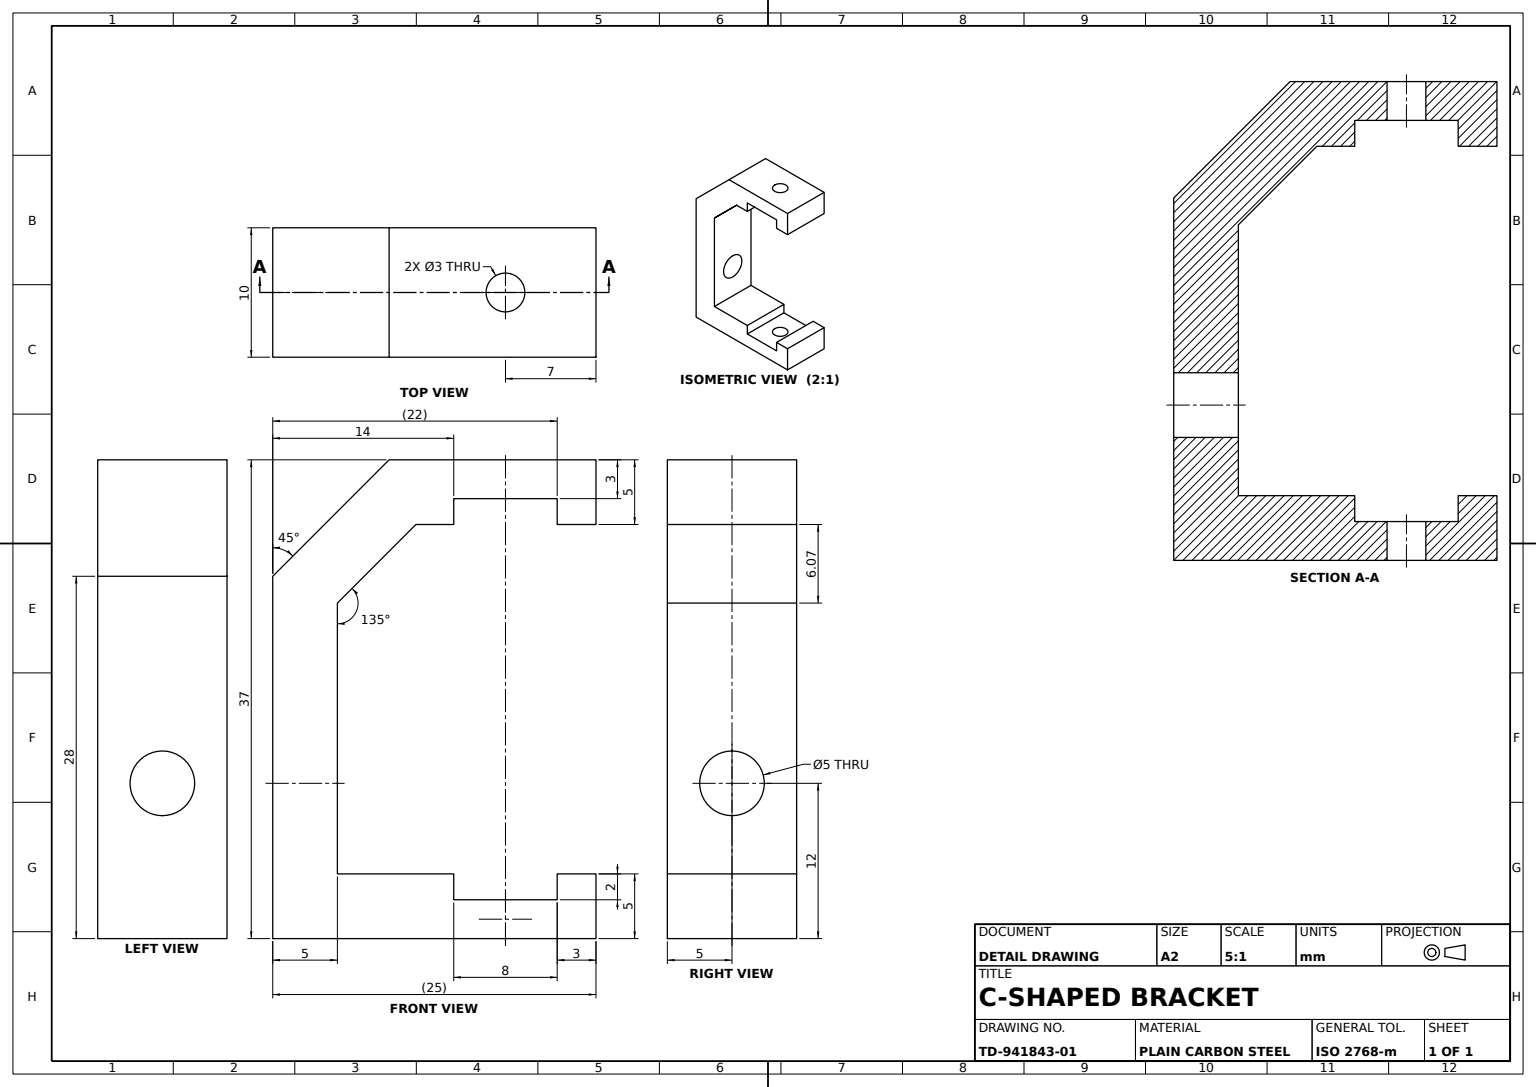
SolidWorks part; units mm, degrees
material "Plain Carbon Steel"
ref_plane "Front Plane" through (0, 0, 0) normal (0, 0, 1) x (1, 0, 0)
ref_plane "Top Plane" through (0, 0, 0) normal (0, 1, 0) x (1, 0, 0)
ref_plane "Right Plane" through (0, 0, 0) normal (1, 0, 0) x (0, 0, -1)
sketch "C Profile Sketch" plane through (0, 0, 0) normal (0, 0, 1) x (1, 0, 0)
  line L0 (0, 0) -> (0, 28)
  line L1 (0, 28) -> (9, 37)
  line L2 (9, 37) -> (25, 37)
  line L3 (25, 37) -> (25, 32)
  line L4 (25, 32) -> (22, 32)
  line L5 (22, 32) -> (22, 34)
  line L6 (22, 34) -> (14, 34)
  line L7 (14, 34) -> (14, 32)
  line L8 (14, 32) -> (11.0711, 32)
  line L9 (11.0711, 32) -> (5, 25.9289)
  line L10 (5, 25.9289) -> (5, 5)
  line L11 (5, 5) -> (14, 5)
  line L12 (14, 5) -> (14, 3)
  line L13 (14, 3) -> (22, 3)
  line L14 (22, 3) -> (22, 5)
  line L15 (22, 5) -> (25, 5)
  line L16 (25, 5) -> (25, 0)
  line L17 (25, 0) -> (0, 0)
  dimension "D1" = 28
  dimension "D2" = 45
  dimension "D3" = 5
  dimension "D4" = 2
  dimension "D5" = 5
  dimension "D6" = 8
  dimension "D7" = 3
  dimension "D8" = 5
  dimension "D9" = 37
  dimension "D10" = 3
  dimension "D11" = 8
  dimension "D12" = 5
  dimension "D13" = 5
  dimension "D14" = 2
  dimension "D15" = 25
  dimension "D16" = 25
  dimension "D17" = 5
extrude "C Bracket Body" add sketch "C Profile Sketch" along normal mid plane 10
sketch "Flange Hole Sketch" plane through (0, 34, 0) normal (0, -1, 0) x (1, 0, 0)
  line L0 (22, 5) -> (22, -5) construction
  line L5 (14, -5) -> (22, -5) construction
  line L6 (0, -5) -> (25, -5) construction
  line L8 (25, 5) -> (25, -5) construction
  circle A0 centre (18, 0) radius 1.5
  dimension "D1" = 3
  dimension "D2" = 5
  dimension "D3" = 7
  dimension "D4" = 4
  dimension "D5" = 5
extrude "Flange Holes Ø3" cut sketch "Flange Hole Sketch" against normal mid plane 200
sketch "Web Hole Sketch" plane through (5, 0, 0) normal (1, 0, 0) x (0, 0, -1)
  line L0 (-5, 0) -> (5, 0) construction
  line L1 (5, 5) -> (5, 25.9289) construction
  circle A0 centre (0, 12) radius 2.5
  dimension "D2" = 5
  dimension "D1" = 12
  dimension "D3" = 5
extrude "Web Hole" cut sketch "Web Hole Sketch" against normal mid plane 200
